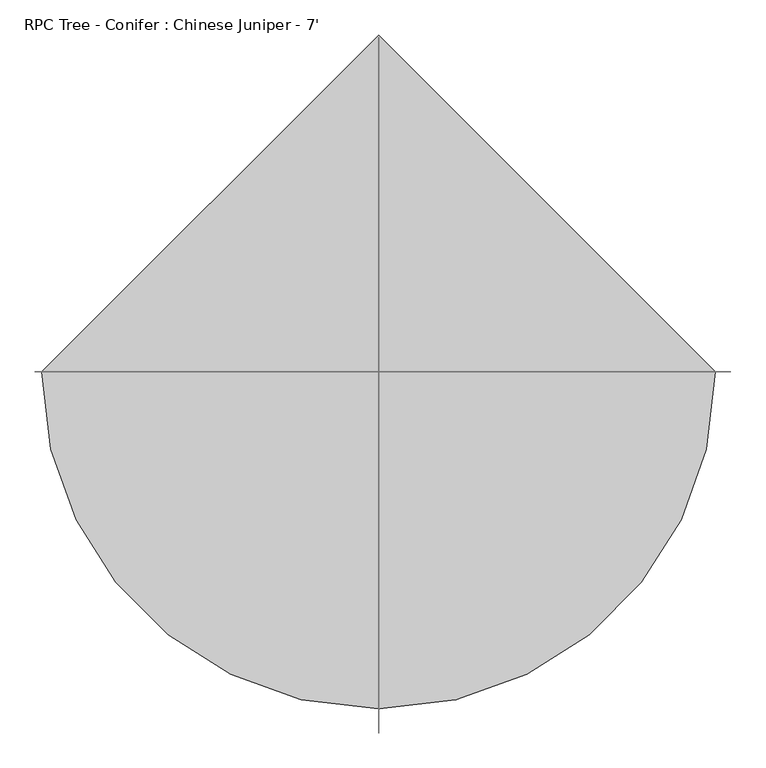
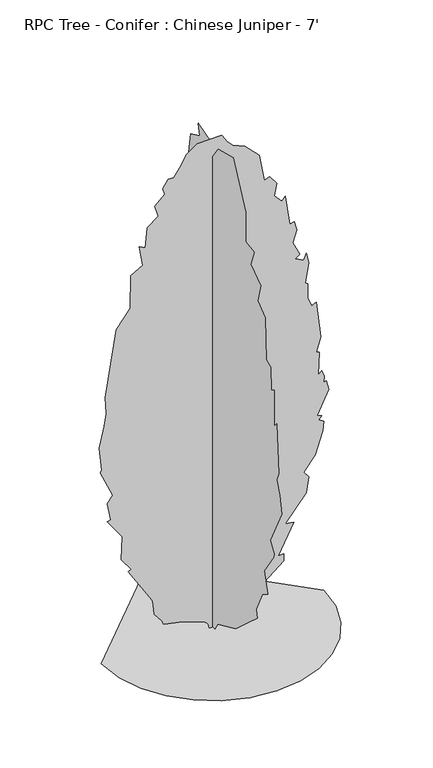
"""IFC4 building model written with IfcOpenShell, lengths in millimetres: geographic element geometry, RPC Tree - Conifer : Chinese Juniper - 7'."""

from ifc_helpers import new_model, si_unit, origin, place, context, project, spatial, triangles, source, transform, mapped, element, save


def rpc_tree_conifer_chinese_juniper_7_2d11b09a(model_context):
    return source(origin(), model_context, "Body", "Tessellation", [
        triangles([(-62.8646902, 2.8e-06, 5.6e-06), (-77.8195323, -1.2e-06, 76.884415), (-118.1706122, -2.6e-06, 130.249081), (-530.2255935, 6.4e-06, 281.8962745), (-864.9722031, 1.68e-05, 352.927949), (-897.0568726, 1.34e-05, 433.1385326), (-1026.3305952, 9.2e-06, 598.6236714), (-1057.4801474, -4.4e-06, 850.2347305), (-1105.6104218, -8.1e-06, 946.4875763), (-1490.61759, -2.76e-05, 1556.0852509), (-1440.8043514, -3.15e-05, 1586.0209236), (-1611.1554359, -3.83e-05, 1824.8325096), (-1593.8906467, -6.43e-05, 2248.4079632), (-1859.5899811, -7.46e-05, 2614.8767281), (-1795.4186073, -7.83e-05, 2630.9115051), (-1857.0972553, -9.5e-05, 2955.0891014), (-1763.3273975, -0.0001065, 3080.0901924), (-1987.9221188, -0.0001263, 3577.4054764), (-1955.8418095, -0.0001296, 3609.4857857), (-2003.9677963, -0.0001534, 4042.6189407), (-1916.9034885, -0.0001797, 4420.5176765), (-1875.6247581, -0.0001943, 4636.1861984), (-1891.6702904, -0.0002118, 4940.9873611), (-1699.1667789, -0.0002919, 6144.1453171), (-1458.5372807, -0.0003216, 6464.992012), (-1445.5287724, -0.0003578, 7063.8281342), (-1233.9425594, -0.0003744, 7186.8915527), (-1298.1139332, -0.0003936, 7555.8527527), (-1188.5924932, -0.0003947, 7493.0205414), (-1153.7363359, -0.0004181, 7860.6539154), (-961.2251215, -0.0004351, 8005.0317307), (-1025.3943878, -0.0004447, 8213.580629), (-848.9298683, -0.000462, 8374.0039764), (-881.0145378, -0.0004673, 8486.3011917), (-784.761692, -0.0004801, 8630.679007), (-688.5087736, -0.0004843, 8630.679007), (-578.0728183, -0.0004977, 8774.066185), (-467.3560298, -0.0005149, 8982.2017365), (-268.711814, -0.0005316, 9116.7167816), (158.4155849, -0.0005507, 9123.4332321), (257.9788208, -0.0005458, 8967.5601883), (354.2317211, -0.0005442, 8871.3085052), (568.2292331, -0.0005482, 8780.6739212), (819.4537605, -0.0005435, 8518.3817917), (915.706679, -0.0005181, 8021.0772629), (1011.9595247, -0.0005242, 8053.1572815), (1129.3535946, -0.0005194, 7885.2123001), (1092.1679283, -0.0005048, 7668.1505493), (1220.5108212, -0.0005018, 7523.7727341), (1284.6714397, -0.0005084, 7587.9438171), (1364.8886364, -0.0004794, 7042.5026917), (1445.0947872, -0.0004839, 7058.5482239), (1488.7139271, -0.0004763, 6899.6271103), (1417.0204834, -0.0004602, 6681.553212), (1541.3466156, -0.0004498, 6416.8658798), (1457.2867756, -0.0004432, 6366.4648865), (1605.5181347, -0.000445, 6288.5231323), (1653.6439762, -0.0004538, 6400.8203476), (1701.7698177, -0.0004444, 6208.3169815), (1637.6091991, -0.0004206, 5855.3902679), (1683.9281742, -0.0004203, 5817.2792221), (1677.4947006, -0.0004045, 5556.6957092), (1749.8958046, -0.0003978, 5390.1657578), (1830.1128559, -0.0004032, 5422.2457764), (1910.3190067, -0.0003665, 4748.4834137), (1830.1128559, -0.0003477, 4491.8083832), (1880.0675102, -0.0003489, 4474.8376167), (1862.1931652, -0.0003233, 4058.664473), (1926.3646843, -0.000329, 4106.7903145), (1974.4905258, -0.0003244, 3994.4930992), (1958.4449936, -0.000317, 3882.2063484), (2006.5708351, -0.0003201, 3898.2411255), (2054.6966766, -0.0003116, 3721.7832916), (1846.1474876, -0.0002777, 3304.6849136), (1926.3646843, -0.0002793, 3272.6046043), (1878.2386974, -0.0002733, 3208.4329399), (1958.4449936, -0.000274, 3160.3070984), (1941.5720409, -0.0002629, 2987.408931), (1814.0671783, -0.0002332, 2582.7853729), (1605.5181347, -0.0002088, 2326.1103424), (1701.7698177, -0.0002063, 2213.8129818), (1649.1590755, -0.0001873, 1933.5703491), (1284.6714397, -0.0001441, 1475.8789547), (1429.0600101, -0.0001495, 1459.8334225), (1156.3393747, -0.000106, 930.4452415), (1252.5911304, -0.0001102, 930.4452415), (1252.5911304, -0.0001026, 802.1077263), (546.7353052, -3.73e-05, 224.5904155), (546.7353052, -4.21e-05, 304.800981), (65.4726297, -2.9e-06, 0.0), (0.1966756, 59.0964473, 0.0005571), (0.1966821, 147.7762179, 61.270002), (0.1966931, 331.812886, 128.3386235), (0.1967019, 764.9514187, 288.7597363), (0.1967208, 989.5417797, 497.3078353), (0.1967173, 893.2889339, 513.35017), (0.1967539, 1236.6210297, 1008.2424551), (0.1967601, 1133.9249725, 1251.2842335), (0.1967737, 1422.6803123, 1668.3826115), (0.1967807, 1390.6000031, 1860.8861229), (0.196801, 1599.1382915, 2117.5612988), (0.1968175, 1669.2534885, 2424.5611645), (0.1968126, 1631.2295013, 2743.2087204), (0.1968406, 1887.9045319, 3128.2160339), (0.1968582, 1903.9393089, 3513.2341026), (0.1968679, 1811.2798485, 3828.3110916), (0.1968788, 1952.0651505, 4331.3850357), (0.1968809, 1823.7331581, 4507.8431602), (0.1968964, 1663.3098106, 5021.193512), (0.1968995, 1775.6071712, 5374.1202255), (0.1969163, 1647.2642784, 5887.4702866), (0.1969226, 1486.8518314, 6192.2714493), (0.1969299, 1406.6347801, 6833.9642578), (0.1969236, 1310.3829517, 6785.838707), (0.1969489, 1310.3829517, 7363.3493866), (0.1969426, 1117.8793676, 7411.4749374), (0.1969359, 1016.0366014, 7754.1586716), (0.1969457, 957.4571829, 8037.1227951), (0.1969457, 764.9514187, 8229.6261612), (0.1969667, 668.6985003, 8807.1478867), (0.1969432, 395.9810987, 8935.4801697), (0.1969541, 437.3992101, 9141.9826813), (0.1969316, 48.637529, 9018.0483856), (0.1969359, 27.0117892, 8742.9762222), (0.1969222, -165.4938592, 9015.6973663), (0.1969074, -630.7159349, 9144.029068), (0.1968735, -1015.7285534, 8357.9584442), (0.1968496, -1015.7285534, 7812.5277832), (0.1968366, -1269.4524559, 7767.3630981), (0.1968286, -1160.1051332, 7475.6466019), (0.1968231, -1469.325721, 7264.5612305), (0.1968121, -1384.6999271, 6930.2165222), (0.1967946, -1609.2838932, 6753.7476425), (0.1967768, -1641.3749577, 5983.7219696), (0.1967686, -1772.3524281, 5927.8457291), (0.1967494, -1785.7527729, 5502.462973), (0.196748, -1882.0044559, 5566.6235916), (0.1967358, -1882.0044559, 4892.8612289), (0.1967193, -1962.2107521, 4989.112912), (0.1966944, -2026.3822712, 4090.7555374), (0.1966908, -1956.7243137, 3937.9523643), (0.1966762, -2058.4733356, 3705.7374687), (0.1966772, -2106.5993225, 3384.8910645), (0.1966618, -1769.7070953, 2695.0828789), (0.1966485, -1882.0044559, 2502.5792221), (0.1966632, -1872.5121574, 2434.6195621), (0.1966573, -1577.2035839, 2005.2746933), (0.1966363, -1689.5009445, 1636.3023022), (0.1966391, -1513.0320648, 1524.0049416), (0.1966472, -1336.5740856, 1138.9977007), (0.1966394, -1368.6543949, 994.6145805), (0.1966409, -1047.8121328, 705.8558979), (0.1966423, -710.9265186, 401.0549532), (0.1966556, -149.4493625, 144.3798682), (0.19667, -69.2408772, 0.0005495), (-1963.3638794, 0.0, 0.0006394), (-1911.4497517, -449.9178137, 0.0006104), (-1763.6103745, -863.0962275, 0.0005793), (-1531.6786011, -1227.6948303, 0.0005474), (-1227.4981853, -1531.875246, 0.000516), (-862.8995825, -1763.8070194, 0.0004862), (-449.7211324, -1911.6463966, 0.0004593), (0.1967593, -1963.5605244, 0.0004366), (450.114495, -1911.6463966, 0.00042), (863.2928724, -1763.8070194, 0.0004108), (1227.8914753, -1531.875246, 0.0004086), (1532.071891, -1227.6948303, 0.0004135), (1764.0036644, -863.0951374, 0.0004251), (1911.8430416, -449.9178137, 0.0004432), (1963.7571693, 0.0001717, 0.0004678), (0.1964146, 1963.5605244, 0.0006707)], [[57, 58, 59], [27, 28, 29], [87, 88, 89], [49, 50, 51], [13, 14, 15], [83, 84, 85], [74, 75, 76], [63, 64, 65], [68, 69, 70], [71, 72, 73], [9, 10, 11], [85, 86, 87], [85, 87, 89], [51, 52, 53], [54, 55, 56], [90, 1, 2], [66, 67, 68], [45, 46, 47], [17, 18, 19], [68, 70, 71], [45, 47, 48], [31, 32, 33], [76, 77, 78], [89, 90, 2], [89, 2, 3], [57, 59, 60], [51, 53, 54], [25, 26, 27], [39, 40, 41], [56, 57, 60], [71, 73, 74], [34, 35, 36], [33, 34, 36], [4, 5, 6], [60, 61, 62], [80, 81, 82], [38, 39, 41], [37, 38, 41], [37, 41, 42], [29, 30, 31], [15, 16, 17], [36, 37, 42], [33, 36, 42], [31, 33, 42], [31, 42, 43], [31, 43, 44], [31, 44, 45], [29, 31, 45], [29, 45, 48], [27, 29, 48], [25, 27, 48], [25, 48, 49], [25, 49, 51], [25, 51, 54], [25, 54, 56], [25, 56, 60], [25, 60, 62], [24, 25, 62], [23, 24, 62], [22, 23, 62], [22, 62, 63], [22, 63, 65], [22, 65, 66], [22, 66, 68], [21, 22, 68], [20, 21, 68], [19, 20, 68], [17, 19, 68], [17, 68, 71], [17, 71, 74], [15, 17, 74], [13, 15, 74], [13, 74, 76], [13, 76, 78], [13, 78, 79], [13, 79, 80], [12, 13, 80], [11, 12, 80], [9, 11, 80], [9, 80, 82], [9, 82, 83], [9, 83, 85], [9, 85, 89], [9, 89, 3], [9, 3, 4], [8, 9, 4], [8, 4, 6], [7, 8, 6], [138, 139, 140], [94, 95, 96], [136, 137, 138], [121, 122, 123], [112, 113, 114], [128, 129, 130], [121, 123, 124], [125, 126, 127], [124, 125, 127], [114, 115, 116], [147, 148, 149], [130, 131, 132], [124, 127, 128], [134, 135, 136], [154, 155, 91], [154, 91, 92], [150, 151, 152], [96, 97, 98], [119, 120, 121], [119, 121, 124], [119, 124, 128], [118, 119, 128], [117, 118, 128], [116, 117, 128], [116, 128, 130], [114, 116, 130], [114, 130, 132], [112, 114, 132], [112, 132, 133], [112, 133, 134], [112, 134, 136], [111, 112, 136], [110, 111, 136], [109, 110, 136], [109, 136, 138], [109, 138, 140], [109, 140, 141], [108, 109, 141], [107, 108, 141], [106, 107, 141], [105, 106, 141], [104, 105, 141], [103, 104, 141], [103, 141, 142], [103, 142, 143], [103, 143, 144], [102, 103, 144], [101, 102, 144], [100, 101, 144], [100, 144, 145], [100, 145, 146], [100, 146, 147], [100, 147, 149], [100, 149, 150], [100, 150, 152], [100, 152, 153], [100, 153, 154], [99, 100, 154], [98, 99, 154], [96, 98, 154], [96, 154, 92], [96, 92, 93], [96, 93, 94], [170, 171, 156], [169, 170, 156], [169, 156, 157], [168, 169, 157], [168, 157, 158], [168, 158, 159], [167, 168, 159], [166, 167, 159], [166, 159, 160], [166, 160, 161], [166, 161, 162], [166, 162, 163], [166, 163, 164], [166, 164, 165]], closed=False),
    ])


if __name__ == "__main__":
    model = new_model("IFC4")
    model_context = context("Model", 3, world=origin())
    ifc_project = project(units=[si_unit("LENGTHUNIT", "METRE", prefix="MILLI")], contexts=[model_context])
    site = spatial("IfcSite", under=ifc_project)
    building = spatial("IfcBuilding", under=site)
    placement = place(None, origin())
    rpc_tree_conifer_chinese_juniper_7_shape = rpc_tree_conifer_chinese_juniper_7_2d11b09a(model_context)
    element("IfcGeographicElement", 1, ObjectType="RPC Tree - Conifer : Chinese Juniper - 7'", at=placement, inside=building, context=model_context, shape_type="MappedRepresentation", body=[
        mapped(rpc_tree_conifer_chinese_juniper_7_shape, transform((0.0, 0.0, 0.0), x_axis=(1.0, 0.0, 0.0), y_axis=(0.0, 1.0, 0.0), z_axis=(0.0, 0.0, 1.0))),
    ])
    save(model, "model.ifc")

# Revit data of these elements
# Type "RPC Tree - Conifer : Chinese Juniper - 7'"
#   built-in parameter 1005198 = "{2, 15},{39, RPC-16-FUM3-UUQ0-UBF0-N000-ST1L-LVER-AU},{1, 0},{1, 0},{2, 35},{1, 8},{5, Color},{1, 0},{1, 0},{3, 0.8},{3, 0.8},{3, 0.8},{1, 8},{7, BBoxMin},{1, 0},{1, 0},{1, 0},{1, 0},{1, 0},{1, 8},{7, BBoxMax},{1, 0},{1, 0},{1, 0},{1, 0},{1, 0},{2, 11},{9, RPCTypeId},{1, 0},{1, 0},{39, RPC-16-FUM3-UUQ0-UBF0-N000-ST1L-LVER-AU},{1, 6},{14, RPCPlantHeight},{1, 0},{1, 0},{1, 7},{2, 11},{7, keyword},{1, 0},{1, 0},{96, :Geometry:RPC:Chinese Juniper:juniperus chinensis:chinese:juniper:cupressaceae:conifer:evergreen},{2, 11},{8, category},{1, 0},{1, 0},{16, :Trees [General]},{2, 11},{12, LocalizedUID},{1, 0},{1, 0},{15, Chinese Juniper},{2, 14},{6, Height},{1, 0},{1, 0},{1, 7},{1, 2},{16, Cast Reflections},{1, 0},{1, 0},{1, 0},{1, 2},{12, Cast Shadows},{1, 0},{1, 0},{1, 1},{1, 2},{9, Lock View},{1, 0},{1, 0},{1, 0},{1, 4},{5, ViewC},{1, 0},{1, 0},{1, 0},{2, 11},{20, AdvancedUIDefinition},{1, 0},{1, 0},{0, },{2, 11},{10, AssetLibID},{1, 0},{1, 0},{36, 4D3F6E72-3F99-4203-98E9-AF80B3C7A7A4},{2, 11},{10, BaseSchema},{1, 0},{1, 0},{9, RPCSchema},{2, 11},{12, ExchangeGUID},{1, 0},{1, 0},{0, },{1, 2},{6, Hidden},{1, 0},{1, 0},{1, 0},{1, 4},{11, RPCCategory},{1, 0},{1, 0},{1, 0},{2, 11},{8, RPCImage},{1, 0},{1, 0},{0, },{1, 4},{13, SchemaVersion},{1, 0},{1, 0},{1, 4},{2, 11},{12, UIDefinition},{1, 0},{1, 0},{0, },{2, 11},{6, UIName},{1, 0},{1, 0},{39, RPC-16-FUM3-UUQ0-UBF0-N000-ST1L-LVER-AU},{2, 11},{11, VersionGUID},{1, 0},{1, 0},{9, RPCSchema},{2, 11},{9, assettype},{1, 0},{1, 0},{11, RPCGeometry},{2, 11},{11, description},{1, 0},{1, 0},{0, },{2, 11},{9, localname},{1, 0},{1, 0},{3, RPC},{2, 11},{9, localtype},{1, 0},{1, 0},{3, RPC},{1, 4},{8, revision},{1, 0},{1, 0},{1, 1},{2, 11},{9, thumbnail},{1, 0},{1, 0},{0, },{1, 4},{7, version},{1, 0},{1, 0},{1, 1},{1, 2},{20, RPC_Cast Reflections},{1, 0},{1, 0},{1, 1},{1, 2},{16, RPC_Cast Shadows},{1, 0},{1, 0},{1, 1},{1, 2},{13, RPC_Lock View},{1, 0},{1, 0},{1, 0},{1, 4},{9, RPC_ViewC},{1, 0},{1, 0},{1, 0},{21, assetlibrary_base.fbx},{1, 5},"
#   built-in parameter 1005195 = "RPC-16-FUM3-UUQ0-UBF0-N000-ST1L-LVER-AU"
#   Type Comments = "Chinese Juniper"
#   Assembly Code = "G2050500"
#   Height = 30' - 0"
#   Description = (empty or 0)
#   Default Elevation = 0
